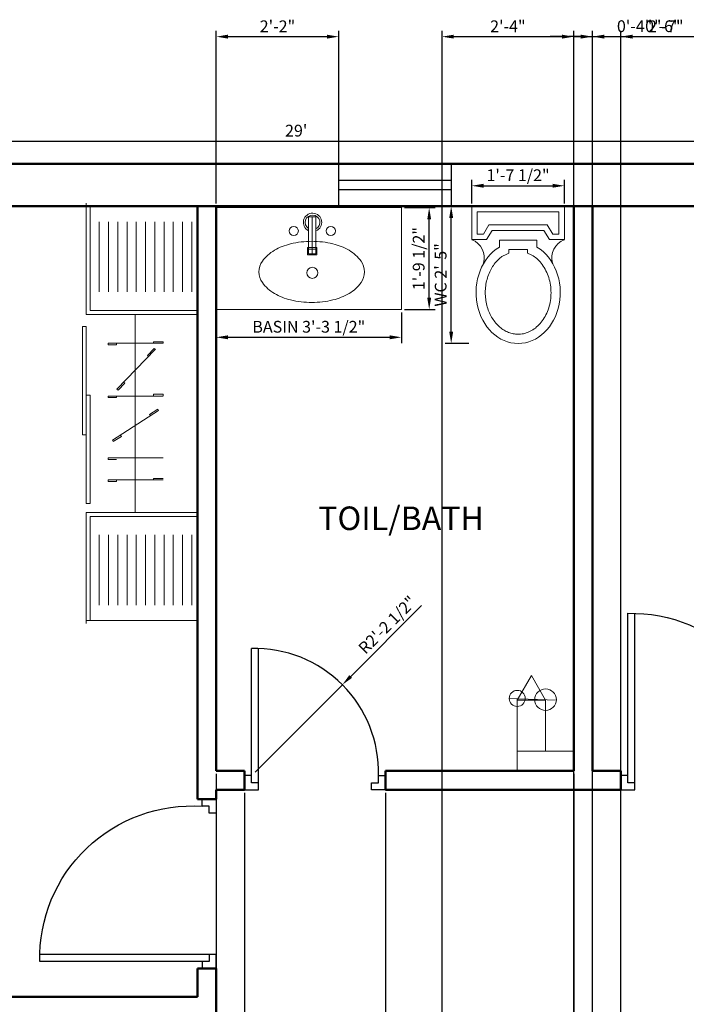
# Model space of a CAD drawing. Units: inches. Extents: x 1905 to 2315, y 3232 to 3824.
# Tile 7 of 8: x 2053 to 2195, y 3615 to 3824. Entities that reach past the tile are written whole.
import ezdxf

# ---------------------------------------------------------------- set-up
doc = ezdxf.new("R2010")
doc.units = ezdxf.units.IN
for name, color, linetype, lineweight in [('A-ANNO-DIMS', 2, 'Continuous', 18), ('A-AREA-IDEN', 7, 'Continuous', 25), ('A-FLOR-CABT', 8, 'Continuous', 18), ('A-FLOR-FIXT', 9, 'Continuous', 18), ('door', 1, 'Continuous', 25), ('wall', 2, 'Continuous', 50), ('WINDOW', 60, 'Continuous', 25)]:
    doc.layers.add(name, color=color, linetype=linetype, lineweight=lineweight)
doc.styles.get("Standard").update_dxf_attribs({"font": 'arial.ttf'})
doc.dimstyles.new('ISO-25', dxfattribs={"dimtxt": 2.5, "dimasz": 2.5, "dimexe": 1.25, "dimexo": 0.625, "dimtad": 1, "dimdec": 1, "dimlunit": 3, "dimtxsty": 'Standard', "dimcen": 2.5, "dimadec": 0, "dimazin": 0, "dimtfac": 1, "dimtdec": 1, "dimtmove": 0, "dimatfit": 3, "dimfxl": 1, "dimarcsym": 0})

# ---------------------------------------------------------------- blocks, each defined once
blk = doc.blocks.new('A$C7C8779AE')
for p, q in [((0, 0.7405), (0, 0.5605)), ((0.5, 0.7405), (0, 0.7405)), ((0.47, 0.7105), (0.03, 0.7105)), ((0.03, 0.7105), (0.03, 0.5905)), ((0.47, 0.5905), (0.47, 0.7105)), ((0.5, 0.5605), (0.5, 0.7405)), ((0.093, 0.6405), (0.063, 0.5905)), ((0.093, 0.6405), (0.407, 0.6405)), ((0.437, 0.5905), (0.407, 0.6405)), ((0.03, 0.5905), (0.063, 0.5905)), ((0.11, 0.6105), (0.08, 0.5605)), ((0.11, 0.6105), (0.39, 0.6105)), ((0.42, 0.5605), (0.39, 0.6105)), ((0.437, 0.5905), (0.47, 0.5905)), ((0, 0.5605), (0.08, 0.5605)), ((0.1497, 0.557), (0.1497, 0.5203)), ((0.1497, 0.557), (0.3514, 0.557)), ((0.3514, 0.557), (0.3514, 0.5203)), ((0.42, 0.5605), (0.5, 0.5605)), ((0.1997, 0.507), (0.1997, 0.4879)), ((0.1997, 0.507), (0.3014, 0.507)), ((0.3014, 0.507), (0.3014, 0.4879))]:
    blk.add_line(p, q)
for centre, start, end in [((-0.0386, 0.4613), 344.642, 68.7339), ((0.5386, 0.4613), 111.2661, 195.358)]:
    blk.add_arc(centre, 0.1064, start, end)
blk.add_ellipse((0.2506, 0.2744), major_axis=(0, 0.2744), ratio=0.828948, start_param=0.459479, end_param=5.823706)
blk.add_open_spline([(0.1997, 0.4879), (0.1697, 0.474), (0.1642, 0.4702), (0.1512, 0.4602), (0.1438, 0.4535), (0.1298, 0.4388), (0.1233, 0.4306), (0.1111, 0.4131), (0.1055, 0.4037), (0.0956, 0.3838), (0.0912, 0.3733), (0.0838, 0.3516), (0.0808, 0.3403), (0.0762, 0.3172), (0.0746, 0.3055), (0.073, 0.2817), (0.0729, 0.2698), (0.0743, 0.246), (0.0758, 0.2342), (0.0801, 0.2111), (0.0831, 0.1998), (0.0903, 0.1779), (0.0945, 0.1673), (0.1043, 0.1473), (0.1098, 0.1378), (0.1218, 0.12), (0.1283, 0.1118), (0.1421, 0.0968), (0.1494, 0.09), (0.1646, 0.078), (0.1725, 0.0728), (0.1887, 0.064), (0.1969, 0.0603), (0.2137, 0.0547), (0.2222, 0.0527), (0.2392, 0.0502), (0.2478, 0.0498), (0.2664, 0.0505), (0.2764, 0.052), (0.2963, 0.0573), (0.3061, 0.061), (0.3253, 0.0707), (0.3346, 0.0766), (0.3525, 0.0906), (0.3611, 0.0987), (0.3771, 0.1169), (0.3845, 0.127), (0.3978, 0.1488), (0.4037, 0.1605), (0.4137, 0.1853), (0.4178, 0.1983), (0.424, 0.2251), (0.4261, 0.2389), (0.4282, 0.2668), (0.4283, 0.2809), (0.4262, 0.3088), (0.4241, 0.3226), (0.418, 0.3495), (0.414, 0.3625), (0.404, 0.3873), (0.3982, 0.3991), (0.385, 0.421), (0.3776, 0.4311), (0.3617, 0.4494), (0.3531, 0.4575), (0.3382, 0.4693), (0.3321, 0.4736), (0.3014, 0.4879)], degree=3, knots=[0.459479, 0.459479, 0.459479, 0.459479, 0.567422, 0.567422, 0.720865, 0.720865, 0.874307, 0.874307, 1.02775, 1.02775, 1.181192, 1.181192, 1.334635, 1.334635, 1.488077, 1.488077, 1.64152, 1.64152, 1.794963, 1.794963, 1.948405, 1.948405, 2.101848, 2.101848, 2.25529, 2.25529, 2.408733, 2.408733, 2.562175, 2.562175, 2.715618, 2.715618, 2.86906, 2.86906, 3.022503, 3.022503, 3.175946, 3.175946, 3.356457, 3.356457, 3.536968, 3.536968, 3.717479, 3.717479, 3.89799, 3.89799, 4.078501, 4.078501, 4.259012, 4.259012, 4.439523, 4.439523, 4.620035, 4.620035, 4.800546, 4.800546, 4.981057, 4.981057, 5.161568, 5.161568, 5.342079, 5.342079, 5.52259, 5.52259, 5.703101, 5.703101, 5.823706, 5.823706, 5.823706, 5.823706])
blk = doc.blocks.new('A$C50A015BB')
for p, q in [((0, 0.55), (1, 0.55)), ((0, 0.55), (0, 0)), ((1, 0.55), (1, 0)), ((0.4985, 0.5), (0.5385, 0.5)), ((0.4985, 0.5), (0.4985, 0.3)), ((0.5185, 0.5), (0.5185, 0.3)), ((0.5385, 0.5), (0.5385, 0.3)), ((0.4935, 0.335), (0.4935, 0.295)), ((0.4935, 0.335), (0.5435, 0.335)), ((0.4985, 0.325), (0.5385, 0.325)), ((0.5435, 0.335), (0.5435, 0.295)), ((0.4935, 0.295), (0.5435, 0.295)), ((0.4985, 0.3), (0.5385, 0.3)), ((0, 0), (1, 0)), ((0, 0), (1, 0))]:
    blk.add_line(p, q)
for centre, radius in [((0.4185, 0.424), 0.025), ((0.6185, 0.424), 0.025), ((0.5185, 0.1981), 0.0298)]:
    blk.add_circle(centre, radius)
for centre, radius, start, end in [((0.5201, 0.4703), 0.0497, 291.7425, 244.2331), ((0.5201, 0.4703), 0.0397, 297.632, 237.0256), ((0.4185, 0.1397), 0.2081, 120.0686, 144.4178), ((0.4772, 0.0383), 0.3252, 103.4853, 120.0686), ((0.5157, -0.1225), 0.4906, 90, 103.4853), ((0.5157, -0.1225), 0.4906, 76.5147, 90), ((0.5543, 0.0383), 0.3252, 59.9314, 76.5147), ((0.613, 0.1397), 0.2081, 35.5822, 59.9314), ((0.3299, 0.2031), 0.0991, 144.4178, 180), ((0.7016, 0.2031), 0.0991, 0, 35.5822), ((0.3299, 0.2031), 0.0991, 180, 215.5822), ((0.7016, 0.2031), 0.0991, 324.4178, 0), ((0.4185, 0.2665), 0.2081, 215.5822, 239.9314), ((0.613, 0.2665), 0.2081, 300.0686, 324.4178), ((0.4772, 0.3679), 0.3252, 239.9314, 256.5147), ((0.5543, 0.3679), 0.3252, 283.4853, 300.0686), ((0.5157, 0.5288), 0.4906, 256.5147, 270), ((0.5157, 0.5288), 0.4906, 270, 283.4853)]:
    blk.add_arc(centre, radius, start, end)
blk = doc.blocks.new('*D15')
at = {"layer": 'A-ANNO-DIMS', "color": 0, "lineweight": -2, "transparency": 16777216}
for p, q in [((1938.01, 3793.86), (1938.01, 3799.33)), ((2286.01, 3793.86), (2286.01, 3799.33)), ((1940.51, 3798.08), (2283.51, 3798.08))]:
    blk.add_line(p, q, dxfattribs=at)
at = {"layer": 'A-ANNO-DIMS', "color": 0, "transparency": 16777216}
for points in [[(1940.51, 3798.5), (1940.51, 3797.67), (1938.01, 3798.08)], [(2283.51, 3798.5), (2283.51, 3797.67), (2286.01, 3798.08)]]:
    blk.add_solid(points, dxfattribs=at)
at = {"layer": 'Defpoints', "color": 0, "transparency": 16777216}
for p in [(2286.01, 3798.08), (1938.01, 3793.23), (2286.01, 3793.23)]:
    blk.add_point(p, dxfattribs=at)
at = {"layer": 'A-ANNO-DIMS', "color": 0, "transparency": 16777216, "insert": (2112.01, 3799.99), "char_height": 2.5, "attachment_point": 5}
blk.add_mtext("29'", dxfattribs=at)
blk = doc.blocks.new('CUPBOARD-DOUBLE-BAY')
at = {"ltscale": 0.05}
for p, q in [((88.68, 24.41), (0.66, 24.41)), ((0.66, 0.79), (0.66, 24.41)), ((88.68, 0.79), (88.68, 24.41)), ((48.39, 17.11), (48.73, 17.11)), ((59.57, 17.11), (59.9, 17.11)), ((30.53, 15.05), (30.86, 15.05)), ((45.28, 16.16), (45.56, 15.98)), ((48.39, 15.05), (48.73, 15.05)), ((58.24, 15.47), (58.47, 15.23)), ((59.57, 15.05), (59.9, 15.05)), ((44.17, 14.43), (44.45, 14.25)), ((56.76, 14.03), (56.99, 13.79)), ((51.32, 8.73), (51.09, 8.97)), ((30.53, 7.22), (30.19, 7.22)), ((38.95, 6.33), (38.67, 6.51)), ((40.06, 8.06), (39.78, 8.24)), ((48.35, 7.22), (48.02, 7.22)), ((49.85, 7.29), (49.61, 7.53)), ((59.57, 7.22), (59.23, 7.22)), ((30.53, 5.41), (30.19, 5.41)), ((35.23, 5.41), (34.9, 5.41)), ((48.35, 5.41), (48.02, 5.41)), ((59.57, 5.41), (59.23, 5.41))]:
    blk.add_line(p, q, dxfattribs=at)
for p, q in [((18.83, 23.23), (3.94, 23.23)), ((22.77, 1.58), (22.77, 24.41)), ((23.62, 0.79), (23.62, 24.41)), ((65.72, 0.79), (65.72, 24.41)), ((66.57, 1.58), (66.57, 24.41)), ((70.51, 23.23), (85.4, 23.23)), ((18.83, 21.26), (3.94, 21.26)), ((70.51, 21.26), (85.4, 21.26)), ((18.83, 19.29), (3.94, 19.29)), ((70.51, 19.29), (85.4, 19.29)), ((18.83, 17.32), (3.94, 17.32)), ((30.53, 5.41), (30.53, 17.11)), ((30.86, 15.05), (30.86, 17.11)), ((35.23, 5.41), (35.23, 17.11)), ((48.35, 5.41), (48.35, 17.11)), ((48.73, 15.05), (48.73, 17.11)), ((59.57, 5.41), (59.57, 17.11)), ((59.9, 15.05), (59.9, 17.11)), ((70.51, 17.32), (85.4, 17.32)), ((18.83, 15.35), (3.94, 15.35)), ((38.95, 6.33), (45.28, 16.16)), ((44.45, 14.25), (45.56, 15.98)), ((49.85, 7.29), (58.22, 15.46)), ((56.99, 13.79), (58.47, 15.23)), ((70.51, 15.35), (85.4, 15.35)), ((18.83, 13.39), (3.94, 13.39)), ((70.51, 13.39), (85.4, 13.39)), ((18.83, 11.42), (3.94, 11.42)), ((65.6, 11.21), (23.75, 11.21)), ((70.51, 11.42), (85.4, 11.42)), ((18.83, 9.45), (3.94, 9.45)), ((49.61, 7.53), (51.09, 8.97)), ((70.51, 9.45), (85.4, 9.45)), ((18.83, 7.48), (3.94, 7.48)), ((30.19, 7.22), (30.19, 5.41)), ((34.9, 7.22), (34.9, 5.41)), ((38.67, 6.51), (39.78, 8.24)), ((48.02, 7.22), (48.02, 5.41)), ((59.23, 7.22), (59.23, 5.41)), ((70.51, 7.48), (85.4, 7.48)), ((18.83, 5.51), (3.94, 5.51)), ((70.51, 5.51), (85.4, 5.51)), ((18.83, 3.54), (3.94, 3.54)), ((70.51, 3.54), (85.4, 3.54)), ((23.62, 0.79), (0, 0.79)), ((22.77, 1.58), (0.66, 1.58)), ((25.54, 1.58), (25.54, 0.79)), ((48.56, 1.58), (25.54, 1.58)), ((25.54, 0.79), (48.56, 0.79)), ((40.11, 0), (40.11, 0.79)), ((40.11, 0.79), (63.12, 0.79)), ((63.12, 0), (40.11, 0)), ((48.56, 0.79), (48.56, 1.58)), ((63.12, 0.79), (63.12, 0)), ((65.72, 0.79), (89.34, 0.79)), ((66.57, 1.58), (88.68, 1.58))]:
    blk.add_line(p, q)
blk = doc.blocks.new('DOOR-SWING-36IN')
for p, q in [((34.51, 36), (37.51, 36)), ((34.51, 34.5), (34.51, 36)), ((37.51, 36), (37.51, 33)), ((36.01, 34.5), (0.01, 34.5)), ((36.01, 34.5), (34.51, 34.5)), ((36.01, 33), (36.01, 34.5)), ((36.01, 33), (0.01, 33)), ((37.51, 33), (36.01, 33)), ((37.51, 3), (36.01, 3)), ((36.01, 3), (36.01, 1.5)), ((37.51, 0), (37.51, 3)), ((36.01, 1.5), (34.51, 1.5)), ((34.51, 1.5), (34.51, 0)), ((34.51, 0), (37.51, 0))]:
    blk.add_line(p, q)
blk.add_arc((32.32, 33.75), 32.32, 178.6705, 273.8756)
blk = doc.blocks.new('WIN-24IN')
for p, q in [((9, 24), (0, 24)), ((0, 24), (0, 0)), ((3.5, 24), (3.5, 0)), ((5.5, 24), (5.5, 0)), ((9, 24), (9, 0)), ((9, 0), (0, 0))]:
    blk.add_line(p, q)
blk = doc.blocks.new('*D35')
at = {"layer": 'A-ANNO-DIMS', "color": 0, "lineweight": -2, "transparency": 16777216}
for p, q in [((2148.71, 3784.23), (2143.71, 3784.23)), ((2144.96, 3757.58), (2144.96, 3781.73)), ((2148.71, 3755.08), (2143.71, 3755.08))]:
    blk.add_line(p, q, dxfattribs=at)
at = {"layer": 'A-ANNO-DIMS', "color": 0, "transparency": 16777216}
for points in [[(2144.54, 3781.73), (2145.38, 3781.73), (2144.96, 3784.23)], [(2144.54, 3757.58), (2145.38, 3757.58), (2144.96, 3755.08)]]:
    blk.add_solid(points, dxfattribs=at)
at = {"layer": 'Defpoints', "color": 0, "transparency": 16777216}
for p in [(2144.96, 3784.23), (2149.33, 3784.23), (2149.33, 3755.08)]:
    blk.add_point(p, dxfattribs=at)
at = {"layer": 'A-ANNO-DIMS', "color": 0, "transparency": 16777216, "insert": (2143.04, 3769.66), "char_height": 2.5, "attachment_point": 5, "rotation": 90}
blk.add_mtext('WC 2\'-5"', dxfattribs=at)
blk = doc.blocks.new('*D36')
at = {"layer": 'A-ANNO-DIMS', "color": 0, "lineweight": -2, "transparency": 16777216}
for p, q in [((2149.33, 3784.86), (2149.33, 3789.85)), ((2169.02, 3784.86), (2169.02, 3789.85)), ((2151.83, 3788.6), (2166.52, 3788.6))]:
    blk.add_line(p, q, dxfattribs=at)
at = {"layer": 'A-ANNO-DIMS', "color": 0, "transparency": 16777216}
for points in [[(2151.83, 3789.02), (2151.83, 3788.19), (2149.33, 3788.6)], [(2166.52, 3789.02), (2166.52, 3788.19), (2169.02, 3788.6)]]:
    blk.add_solid(points, dxfattribs=at)
at = {"layer": 'Defpoints', "color": 0, "transparency": 16777216}
for p in [(2169.02, 3788.6), (2149.33, 3784.23), (2169.02, 3784.23)]:
    blk.add_point(p, dxfattribs=at)
at = {"layer": 'A-ANNO-DIMS', "color": 0, "transparency": 16777216, "insert": (2159.17, 3790.52), "char_height": 2.5, "attachment_point": 5}
blk.add_mtext('1\'-7 1/2"', dxfattribs=at)
blk = doc.blocks.new('*D37')
at = {"layer": 'A-ANNO-DIMS', "color": 0, "lineweight": -2, "transparency": 16777216}
for p, q in [((2095.01, 3761.67), (2095.01, 3755.14)), ((2134.38, 3761.67), (2134.38, 3755.14)), ((2097.51, 3756.39), (2131.88, 3756.39))]:
    blk.add_line(p, q, dxfattribs=at)
at = {"layer": 'A-ANNO-DIMS', "color": 0, "transparency": 16777216}
for points in [[(2097.51, 3756.81), (2097.51, 3755.97), (2095.01, 3756.39)], [(2131.88, 3756.81), (2131.88, 3755.97), (2134.38, 3756.39)]]:
    blk.add_solid(points, dxfattribs=at)
at = {"layer": 'Defpoints', "color": 0, "transparency": 16777216}
for p in [(2095.01, 3762.3), (2134.38, 3762.3), (2134.38, 3756.39)]:
    blk.add_point(p, dxfattribs=at)
at = {"layer": 'A-ANNO-DIMS', "color": 0, "transparency": 16777216, "insert": (2114.69, 3758.31), "char_height": 2.5, "attachment_point": 5}
blk.add_mtext('BASIN 3\'-3 1/2"', dxfattribs=at)
blk = doc.blocks.new('*D38')
at = {"layer": 'A-ANNO-DIMS', "color": 0, "lineweight": -2, "transparency": 16777216}
for p, q in [((2135, 3783.95), (2141.53, 3783.95)), ((2140.28, 3764.8), (2140.28, 3781.45)), ((2135, 3762.3), (2141.53, 3762.3))]:
    blk.add_line(p, q, dxfattribs=at)
at = {"layer": 'A-ANNO-DIMS', "color": 0, "transparency": 16777216}
for points in [[(2139.87, 3781.45), (2140.7, 3781.45), (2140.28, 3783.95)], [(2139.87, 3764.8), (2140.7, 3764.8), (2140.28, 3762.3)]]:
    blk.add_solid(points, dxfattribs=at)
at = {"layer": 'Defpoints', "color": 0, "transparency": 16777216}
for p in [(2134.38, 3783.95), (2140.28, 3783.95), (2134.38, 3762.3)]:
    blk.add_point(p, dxfattribs=at)
at = {"layer": 'A-ANNO-DIMS', "color": 0, "transparency": 16777216, "insert": (2138.37, 3773.12), "char_height": 2.5, "attachment_point": 5, "rotation": 90}
blk.add_mtext('1\'-9 1/2"', dxfattribs=at)
blk = doc.blocks.new('*D40')
at = {"layer": 'A-ANNO-DIMS', "color": 0, "lineweight": -2, "transparency": 16777216}
for p, q in [((2095.01, 3784.86), (2095.01, 3821.54)), ((2121.05, 3784.86), (2121.05, 3821.54)), ((2097.51, 3820.29), (2118.55, 3820.29))]:
    blk.add_line(p, q, dxfattribs=at)
at = {"layer": 'A-ANNO-DIMS', "color": 0, "transparency": 16777216}
for points in [[(2097.51, 3820.71), (2097.51, 3819.88), (2095.01, 3820.29)], [(2118.55, 3820.71), (2118.55, 3819.88), (2121.05, 3820.29)]]:
    blk.add_solid(points, dxfattribs=at)
at = {"layer": 'Defpoints', "color": 0, "transparency": 16777216}
for p in [(2121.05, 3820.29), (2095.01, 3784.23), (2121.05, 3784.23)]:
    blk.add_point(p, dxfattribs=at)
at = {"layer": 'A-ANNO-DIMS', "color": 0, "transparency": 16777216, "insert": (2108.03, 3822.17), "char_height": 2.5, "attachment_point": 5}
blk.add_mtext('2\'-2"', dxfattribs=at)
blk = doc.blocks.new('*D41')
at = {"layer": 'A-ANNO-DIMS', "color": 0, "lineweight": -2, "transparency": 16777216}
for p, q in [((2095.01, 3663.61), (2095.01, 3232.16)), ((2171.01, 3663.61), (2171.01, 3232.16)), ((2097.51, 3233.41), (2168.51, 3233.41))]:
    blk.add_line(p, q, dxfattribs=at)
at = {"layer": 'A-ANNO-DIMS', "color": 0, "transparency": 16777216}
for points in [[(2097.51, 3233.83), (2097.51, 3233), (2095.01, 3233.41)], [(2168.51, 3233.83), (2168.51, 3233), (2171.01, 3233.41)]]:
    blk.add_solid(points, dxfattribs=at)
at = {"layer": 'Defpoints', "color": 0, "transparency": 16777216}
for p in [(2095.01, 3664.23), (2171.01, 3664.23), (2171.01, 3233.41)]:
    blk.add_point(p, dxfattribs=at)
at = {"layer": 'A-ANNO-DIMS', "color": 0, "transparency": 16777216, "insert": (2133.01, 3235.31), "char_height": 2.5, "attachment_point": 5}
blk.add_mtext('6\'-4"', dxfattribs=at)
blk = doc.blocks.new('*D42')
at = {"layer": 'A-ANNO-DIMS', "color": 0, "lineweight": -2, "transparency": 16777216}
for p, q in [((2175.01, 3784.86), (2175.01, 3821.54)), ((2206.15, 3784.86), (2206.15, 3821.54)), ((2177.51, 3820.29), (2203.65, 3820.29))]:
    blk.add_line(p, q, dxfattribs=at)
at = {"layer": 'A-ANNO-DIMS', "color": 0, "transparency": 16777216}
for points in [[(2177.51, 3820.71), (2177.51, 3819.88), (2175.01, 3820.29)], [(2203.65, 3820.71), (2203.65, 3819.88), (2206.15, 3820.29)]]:
    blk.add_solid(points, dxfattribs=at)
at = {"layer": 'Defpoints', "color": 0, "transparency": 16777216}
for p in [(2206.15, 3820.29), (2175.01, 3784.23), (2206.15, 3784.23)]:
    blk.add_point(p, dxfattribs=at)
at = {"layer": 'A-ANNO-DIMS', "color": 0, "transparency": 16777216, "insert": (2190.58, 3822.17), "char_height": 2.5, "attachment_point": 5}
blk.add_mtext('2\'-7"', dxfattribs=at)
blk = doc.blocks.new('*D63')
at = {"layer": 'A-ANNO-DIMS', "color": 0, "lineweight": -2, "transparency": 16777216}
for p, q in [((2171.01, 3480.07), (2171.01, 3821.54)), ((2175.01, 3476.07), (2175.01, 3821.54)), ((2168.51, 3820.29), (2166.01, 3820.29)), ((2171.01, 3820.29), (2175.01, 3820.29)), ((2177.51, 3820.29), (2187.9, 3820.29))]:
    blk.add_line(p, q, dxfattribs=at)
at = {"layer": 'A-ANNO-DIMS', "color": 0, "transparency": 16777216}
for points in [[(2168.51, 3820.71), (2168.51, 3819.88), (2171.01, 3820.29)], [(2177.51, 3820.71), (2177.51, 3819.88), (2175.01, 3820.29)]]:
    blk.add_solid(points, dxfattribs=at)
at = {"layer": 'Defpoints', "color": 0, "transparency": 16777216}
for p in [(2175.01, 3820.29), (2171.01, 3479.45), (2175.01, 3475.45)]:
    blk.add_point(p, dxfattribs=at)
at = {"layer": 'A-ANNO-DIMS', "color": 0, "transparency": 16777216, "insert": (2183.96, 3822.19), "char_height": 2.5, "attachment_point": 5}
blk.add_mtext('0\'-4"', dxfattribs=at)
blk = doc.blocks.new('*D64')
at = {"layer": 'A-ANNO-DIMS', "color": 0, "lineweight": -2, "transparency": 16777216}
for p, q in [((2101.01, 3659.61), (2101.01, 3232.16)), ((2131.01, 3659.61), (2131.01, 3232.16)), ((2103.51, 3233.41), (2128.51, 3233.41))]:
    blk.add_line(p, q, dxfattribs=at)
at = {"layer": 'A-ANNO-DIMS', "color": 0, "transparency": 16777216}
for points in [[(2103.51, 3233.83), (2103.51, 3233), (2101.01, 3233.41)], [(2128.51, 3233.83), (2128.51, 3233), (2131.01, 3233.41)]]:
    blk.add_solid(points, dxfattribs=at)
at = {"layer": 'Defpoints', "color": 0, "transparency": 16777216}
for p in [(2101.01, 3660.23), (2131.01, 3660.23), (2131.01, 3233.41)]:
    blk.add_point(p, dxfattribs=at)
at = {"layer": 'A-ANNO-DIMS', "color": 0, "transparency": 16777216, "insert": (2116.01, 3235.31), "char_height": 2.5, "attachment_point": 5}
blk.add_mtext('2\'-6"', dxfattribs=at)
blk = doc.blocks.new('*D65')
at = {"layer": 'A-ANNO-DIMS', "color": 0, "lineweight": -2, "transparency": 16777216}
for p, q in [((2095.01, 3659.61), (2095.01, 3232.16)), ((2101.01, 3659.61), (2101.01, 3232.16)), ((2092.51, 3233.41), (2090.01, 3233.41)), ((2095.01, 3233.41), (2101.01, 3233.41)), ((2103.51, 3233.41), (2113.9, 3233.41))]:
    blk.add_line(p, q, dxfattribs=at)
at = {"layer": 'A-ANNO-DIMS', "color": 0, "transparency": 16777216}
for points in [[(2092.51, 3233.83), (2092.51, 3233), (2095.01, 3233.41)], [(2103.51, 3233.83), (2103.51, 3233), (2101.01, 3233.41)]]:
    blk.add_solid(points, dxfattribs=at)
at = {"layer": 'Defpoints', "color": 0, "transparency": 16777216}
for p in [(2095.01, 3660.23), (2101.01, 3660.23), (2101.01, 3233.41)]:
    blk.add_point(p, dxfattribs=at)
at = {"layer": 'A-ANNO-DIMS', "color": 0, "transparency": 16777216, "insert": (2109.96, 3235.31), "char_height": 2.5, "attachment_point": 5}
blk.add_mtext('0\'-6"', dxfattribs=at)
blk = doc.blocks.new('*D70')
at = {"layer": 'A-ANNO-DIMS', "color": 0, "lineweight": -2, "transparency": 16777216}
for p, q in [((2175.01, 3476.07), (2175.01, 3821.54)), ((2181.01, 3476.07), (2181.01, 3821.54)), ((2172.51, 3820.29), (2170.01, 3820.29)), ((2175.01, 3820.29), (2181.01, 3820.29)), ((2183.51, 3820.29), (2193.9, 3820.29))]:
    blk.add_line(p, q, dxfattribs=at)
at = {"layer": 'A-ANNO-DIMS', "color": 0, "transparency": 16777216}
for points in [[(2172.51, 3820.71), (2172.51, 3819.88), (2175.01, 3820.29)], [(2183.51, 3820.71), (2183.51, 3819.88), (2181.01, 3820.29)]]:
    blk.add_solid(points, dxfattribs=at)
at = {"layer": 'Defpoints', "color": 0, "transparency": 16777216}
for p in [(2181.01, 3820.29), (2175.01, 3475.45), (2181.01, 3475.45)]:
    blk.add_point(p, dxfattribs=at)
at = {"layer": 'A-ANNO-DIMS', "color": 0, "transparency": 16777216, "insert": (2189.96, 3822.19), "char_height": 2.5, "attachment_point": 5}
blk.add_mtext('0\'-6"', dxfattribs=at)
blk = doc.blocks.new('*D72')
at = {"layer": 'A-ANNO-DIMS', "color": 0, "lineweight": -2, "transparency": 16777216}
for p, q in [((2143.01, 3373.22), (2143.01, 3821.54)), ((2171.01, 3373.22), (2171.01, 3821.54)), ((2145.51, 3820.29), (2168.51, 3820.29))]:
    blk.add_line(p, q, dxfattribs=at)
at = {"layer": 'A-ANNO-DIMS', "color": 0, "transparency": 16777216}
for points in [[(2145.51, 3820.71), (2145.51, 3819.88), (2143.01, 3820.29)], [(2168.51, 3820.71), (2168.51, 3819.88), (2171.01, 3820.29)]]:
    blk.add_solid(points, dxfattribs=at)
at = {"layer": 'Defpoints', "color": 0, "transparency": 16777216}
for p in [(2171.01, 3820.29), (2143.01, 3372.6), (2171.01, 3372.6)]:
    blk.add_point(p, dxfattribs=at)
at = {"layer": 'A-ANNO-DIMS', "color": 0, "transparency": 16777216, "insert": (2157.01, 3822.17), "char_height": 2.5, "attachment_point": 5}
blk.add_mtext('2\'-4"', dxfattribs=at)
blk = doc.blocks.new('*D73')
at = {"layer": 'A-ANNO-DIMS', "color": 0, "lineweight": -2, "transparency": 16777216}
for p, q in [((2138.67, 3699.39), (2123.59, 3684.32)), ((2103.26, 3663.98), (2121.83, 3682.55))]:
    blk.add_line(p, q, dxfattribs=at)
at = {"layer": 'A-ANNO-DIMS', "color": 0, "transparency": 16777216}
blk.add_solid([(2123.3, 3684.61), (2123.89, 3684.02), (2121.83, 3682.55)], dxfattribs=at)
at = {"layer": 'Defpoints', "color": 0, "transparency": 16777216}
for p in [(2121.83, 3682.55), (2103.26, 3663.98)]:
    blk.add_point(p, dxfattribs=at)
at = {"layer": 'A-ANNO-DIMS', "color": 0, "transparency": 16777216, "insert": (2131.61, 3695.05), "char_height": 2.5, "attachment_point": 5, "rotation": 44.9997}
blk.add_mtext('R2\'-2 1/2"', dxfattribs=at)

msp = doc.modelspace()

# ---------------------------------------------------------------- linework, layer by layer
at = {"layer": 'A-FLOR-FIXT'}
for p, q in [((2157.28, 3679.65), (2167.32, 3679.3)), ((2159, 3668.42), (2159, 3679.65)), ((2165, 3668.42), (2165.03, 3679.38))]:
    msp.add_line(p, q, dxfattribs=at)
for points in [[(2159, 3679.3), (2165.03, 3679.28), (2162.03, 3684.52)], [(2171.01, 3664.23), (2159, 3664.23), (2159, 3668.42), (2171.01, 3668.42)]]:
    msp.add_lwpolyline(points, close=True, dxfattribs=at)
for centre, radius in [((2159, 3679.65), 1.71), ((2165.03, 3679.38), 2.3)]:
    msp.add_circle(centre, radius, dxfattribs=at)
at = {"layer": 'door'}
for p, q in [((2102.51, 3661.73), (2102.51, 3690.23)), ((2104.01, 3660.23), (2104.01, 3690.23)), ((2101.01, 3663.23), (2101.01, 3660.23)), ((2102.51, 3663.23), (2101.01, 3663.23)), ((2102.51, 3661.73), (2102.51, 3663.23)), ((2129.51, 3661.73), (2129.51, 3663.23)), ((2129.51, 3663.23), (2131.01, 3663.23)), ((2131.01, 3663.23), (2131.01, 3660.23)), ((2101.01, 3660.23), (2104.01, 3660.23)), ((2104.01, 3661.73), (2102.51, 3661.73)), ((2104.01, 3660.23), (2104.01, 3661.73)), ((2128.01, 3660.23), (2128.01, 3661.73)), ((2128.01, 3661.73), (2129.51, 3661.73)), ((2131.01, 3660.23), (2128.01, 3660.23))]:
    msp.add_line(p, q, dxfattribs=at)
msp.add_arc((2103.26, 3663.98), 26.26, 358.3634, 91.6366, dxfattribs=at)
at = {"layer": 'wall'}
for p, q in [((2286.01, 3793.23), (1938.01, 3793.23)), ((2277.01, 3784.23), (1947.01, 3784.23)), ((2091.01, 3784.23), (2091.01, 3658.23)), ((2095.01, 3784.23), (2095.01, 3664.23)), ((2171.01, 3664.23), (2171.01, 3784.23)), ((2175.01, 3664.23), (2175.01, 3784.23)), ((2101.01, 3664.23), (2095.01, 3664.23)), ((2101.01, 3664.23), (2101.01, 3660.23)), ((2171.01, 3664.23), (2131.01, 3664.23)), ((2131.01, 3664.23), (2131.01, 3660.23)), ((2181.01, 3664.23), (2175.01, 3664.23)), ((2181.01, 3664.23), (2181.01, 3660.23)), ((2095.01, 3660.23), (2095.01, 3658.23)), ((2101.01, 3660.23), (2095.01, 3660.23)), ((2181.01, 3660.23), (2131.01, 3660.23)), ((2091.01, 3658.23), (2095.01, 3658.23)), ((2091.01, 3622.23), (2095.01, 3622.23)), ((2091.01, 3622.23), (2091.01, 3616.23)), ((2095.01, 3622.23), (2095.01, 3606.23)), ((2091.01, 3616.23), (1947.01, 3616.23))]:
    msp.add_line(p, q, dxfattribs=at)

# ---------------------------------------------------------------- block references
at = {"layer": 'A-FLOR-CABT', "extrusion": (0, 0, -1), "zscale": -1, "rotation": 90.0000000000057}
msp.add_blockref('CUPBOARD-DOUBLE-BAY', (-2066.6, 3695.55), dxfattribs=at)
at = {"layer": 'A-FLOR-FIXT', "xscale": 39.37007874015748, "yscale": 39.37007874015748, "zscale": 39.37007874015748}
for name, p in [('A$C50A015BB', (2095.01, 3762.3)), ('A$C7C8779AE', (2149.33, 3755.08))]:
    msp.add_blockref(name, p, dxfattribs=at)
at = {"layer": 'door', "extrusion": (0, 0, -1), "zscale": -1}
for p, rotation in [((-2217.01, 3697.74), 270.0000000000044), ((-2057.5, 3658.23), 180)]:
    msp.add_blockref('DOOR-SWING-36IN', p, dxfattribs=dict(at, rotation=rotation))
at = {"layer": 'WINDOW', "rotation": 270.0000000000038}
msp.add_blockref('WIN-24IN', (2121.05, 3793.23), dxfattribs=at)

# ---------------------------------------------------------------- texts
at = {"layer": 'A-AREA-IDEN', "insert": (2116.7, 3720.43), "char_height": 5, "attachment_point": 1}
msp.add_mtext_dynamic_manual_height_columns('TOIL/BATH', width=56.1502, gutter_width=12.5, heights=[0], dxfattribs=at)

# ---------------------------------------------------------------- dimensions: what is measured, and where the dimension line sits
at = {"layer": 'A-ANNO-DIMS'}
for base, p1, p2, override, picture, middle in [((2121.05, 3820.29), (2095.01, 3784.23), (2121.05, 3784.23), {"dimdec": 1, "dimlfac": 1, "dimrnd": 0, "dimzin": 1, "dimdsep": 46, "dimlunit": 4, "dimfrac": 2}, '*D40', (2108.03, 3822.17)), ((2171.01, 3820.29), (2143.01, 3372.6), (2171.01, 3372.6), {"dimdec": 1, "dimlfac": 1, "dimrnd": 0, "dimzin": 1, "dimdsep": 46, "dimlunit": 4, "dimfrac": 2}, '*D72', (2157.01, 3822.17)), ((2175.01, 3820.29), (2171.01, 3479.45), (2175.01, 3475.45), {"dimdec": 1, "dimlfac": 1, "dimrnd": 0, "dimzin": 1, "dimdsep": 46, "dimlunit": 4, "dimfrac": 2}, '*D63', (2183.96, 3822.19)), ((2181.01, 3820.29), (2175.01, 3475.45), (2181.01, 3475.45), {"dimdec": 1, "dimlfac": 1, "dimrnd": 0, "dimzin": 1, "dimdsep": 46, "dimlunit": 4, "dimfrac": 2}, '*D70', (2189.96, 3822.19)), ((2206.15, 3820.29), (2175.01, 3784.23), (2206.15, 3784.23), {"dimdec": 1, "dimlfac": 1, "dimrnd": 0, "dimzin": 1, "dimdsep": 46, "dimlunit": 4, "dimfrac": 2}, '*D42', (2190.58, 3822.17)), ((2286.01, 3798.08), (1938.01, 3793.23), (2286.01, 3793.23), {"dimclrd": 0, "dimclre": 0, "dimclrt": 0}, '*D15', (2112.01, 3799.99)), ((2169.02, 3788.6), (2149.33, 3784.23), (2169.02, 3784.23), {"dimdec": 1, "dimlfac": 1, "dimrnd": 0, "dimzin": 1, "dimdsep": 46, "dimlunit": 4, "dimfrac": 2}, '*D36', (2159.17, 3790.52)), ((2171.01, 3233.41), (2095.01, 3664.23), (2171.01, 3664.23), {"dimdec": 1, "dimlfac": 1, "dimrnd": 0, "dimzin": 1, "dimdsep": 46, "dimlunit": 4, "dimfrac": 2}, '*D41', (2133.01, 3235.31)), ((2101.01, 3233.41), (2095.01, 3660.23), (2101.01, 3660.23), {"dimdec": 1, "dimlfac": 1, "dimrnd": 0, "dimzin": 1, "dimdsep": 46, "dimlunit": 4, "dimfrac": 2}, '*D65', (2109.96, 3235.31)), ((2131.01, 3233.41), (2101.01, 3660.23), (2131.01, 3660.23), {"dimdec": 1, "dimlfac": 1, "dimrnd": 0, "dimzin": 1, "dimdsep": 46, "dimlunit": 4, "dimfrac": 2}, '*D64', (2116.01, 3235.31))]:
    dim = msp.add_linear_dim(base=base, p1=p1, p2=p2, dimstyle='ISO-25', override=override, dxfattribs=at)
    dim.commit()
    dim.dimension.update_dxf_attribs({"geometry": picture, "text_midpoint": middle})
dim = msp.add_linear_dim(base=(2140.2832, 3783.9491), p1=(2134.3777, 3762.2956), p2=(2134.3777, 3783.9491), angle=90, dimstyle='ISO-25', override={"dimdec": 1, "dimlfac": 1, "dimrnd": 0, "dimzin": 1, "dimdsep": 46, "dimlunit": 4, "dimfrac": 2}, dxfattribs=at)
dim.commit()
dim.dimension.update_dxf_attribs({"geometry": '*D38', "text_midpoint": (2138.3656, 3773.1224)})
dim = msp.add_linear_dim(base=(2144.9595, 3784.2318), p1=(2149.3323, 3755.0798), p2=(2149.3323, 3784.2318), angle=90, text='WC <>', dimstyle='ISO-25', override={"dimdec": 1, "dimlfac": 1, "dimrnd": 0, "dimzin": 1, "dimdsep": 46, "dimlunit": 4, "dimfrac": 2}, dxfattribs=at)
dim.commit()
dim.dimension.update_dxf_attribs({"geometry": '*D35', "text_midpoint": (2143.0418, 3769.6558)})
dim = msp.add_linear_dim(base=(2134.38, 3756.39), p1=(2095.01, 3762.3), p2=(2134.38, 3762.3), text='BASIN <>', dimstyle='ISO-25', override={"dimdec": 1, "dimlfac": 1, "dimrnd": 0, "dimzin": 1, "dimdsep": 46, "dimlunit": 4, "dimfrac": 2}, dxfattribs=at)
dim.commit()
dim.dimension.update_dxf_attribs({"geometry": '*D37', "text_midpoint": (2114.69, 3758.31)})
dim = msp.add_radius_dim(center=(2103.26, 3663.98), mpoint=(2121.83, 3682.55), dimstyle='ISO-25', override={"dimdec": 1, "dimlfac": 1, "dimrnd": 0, "dimzin": 1, "dimdsep": 46, "dimlunit": 4, "dimfrac": 2}, dxfattribs=at)
dim.commit()
dim.dimension.update_dxf_attribs({"geometry": '*D73', "text_midpoint": (2132.97, 3693.69), "dimtype": 164})

doc.saveas('drawing.dxf')
